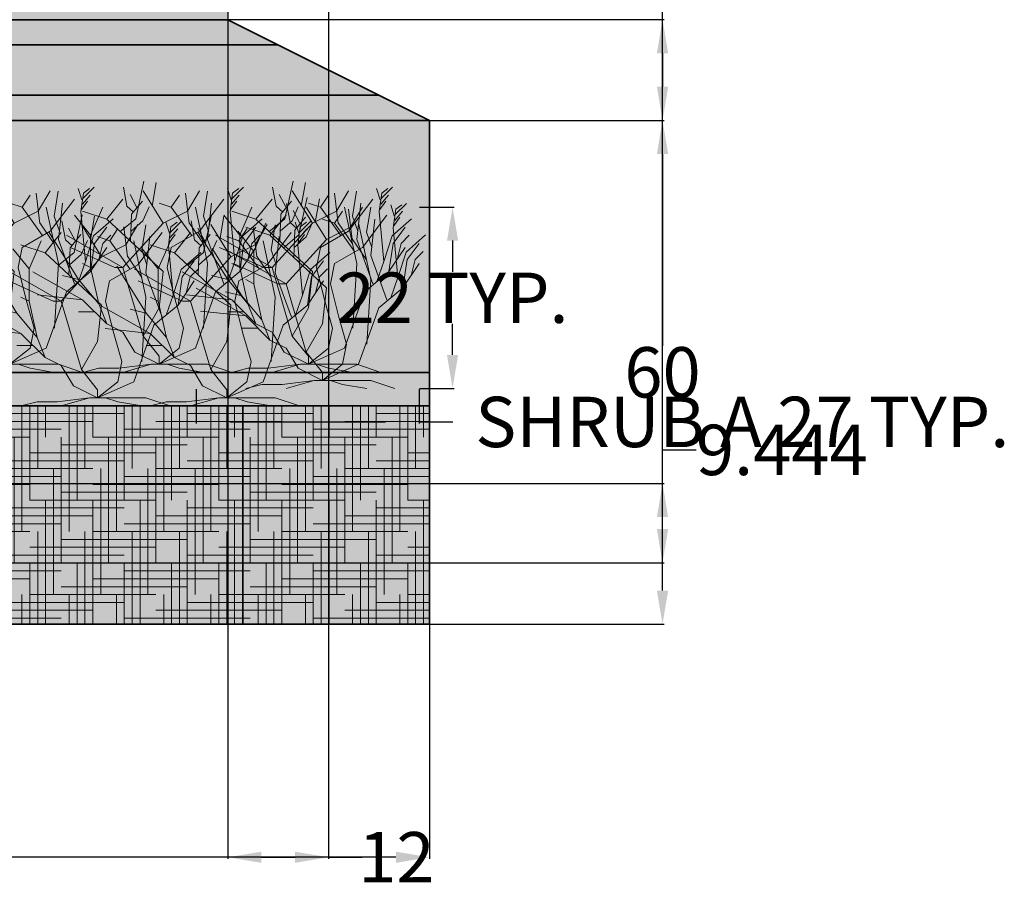
# Model space of a CAD drawing. Units: inches. Extents: x 221 to 874, y 171 to 738.
# Tile 9 of 11: x 756 to 874, y 171 to 275. Entities that reach past the tile are written whole.
import ezdxf

# ---------------------------------------------------------------- set-up
doc = ezdxf.new("R2010")
doc.units = ezdxf.units.IN
doc.header["$MEASUREMENT"] = 0
for name, color, linetype, lineweight in [('A-ANNO-DIMS', 2, 'Continuous', 18), ('A-ELEV', 7, 'Continuous', 35), ('A-ELEV-PATT', 8, 'Continuous', 13), ('L-PLNT', 3, 'Continuous', 13)]:
    doc.layers.add(name, color=color, linetype=linetype, lineweight=lineweight)
doc.styles.get("Standard").update_dxf_attribs({"font": 'arial.ttf'})
doc.dimstyles.get("Standard").update_dxf_attribs({"dimtxt": 6, "dimasz": 4, "dimexe": 0.18, "dimexo": 0.0625, "dimgap": 0.09, "dimtad": 0, "dimtih": 1, "dimtoh": 1, "dimdec": 0, "dimzin": 0, "dimdsep": 46, "dimlunit": 3, "dimtxsty": 'Standard', "dimcen": 0.09, "dimadec": 0, "dimazin": 0, "dimtfac": 1, "dimtdec": 0, "dimtofl": 0, "dimtmove": 0, "dimatfit": 3, "dimfxl": 1, "dimtolj": 1, "dimtzin": 0, "dimarcsym": 0})

# ---------------------------------------------------------------- blocks, each defined once
blk = doc.blocks.new('SHRUB-A')
for p, q in [((15.5, 17.76), (13.1, 21.6)), ((18.38, 19.2), (19.82, 21.6)), ((8.78, 18.24), (10.7, 20.64)), ((19.82, 16.8), (22.7, 20.64)), ((8.78, 18.24), (5.9, 19.2)), ((6.86, 16.32), (8.3, 19.68)), ((15.5, 17.76), (18.38, 19.2)), ((6.86, 16.32), (4.94, 18.72)), ((15.5, 12), (8.78, 18.24)), ((10.7, 12.48), (15.5, 17.76)), ((5.42, 11.04), (1.91, 16.66)), ((16.46, 14.88), (19.82, 16.8)), ((25.1, 15.36), (26.54, 17.28)), ((10.7, 12.48), (3.98, 16.32)), ((6.86, 12.48), (6.86, 16.32)), ((24.62, 12), (25.1, 15.36)), ((9.74, 12.48), (4.46, 14.88)), ((15.98, 12.48), (16.46, 14.88)), ((24.62, 12), (26.54, 14.88)), ((6.86, 12.48), (5.9, 12.96)), ((5.9, 8.64), (0, 11.96)), ((7.82, 8.16), (6.86, 12.48)), ((10.7, 12.48), (9.74, 12.48)), ((13.1, 4.32), (10.7, 12.48)), ((15.02, 7.68), (15.5, 12)), ((16.94, 8.64), (15.98, 12.48)), ((21.74, 9.6), (24.62, 12)), ((5.42, 11.04), (3.5, 11.52)), ((7.82, 8.16), (5.42, 11.04)), ((19.34, 2.88), (21.74, 9.6)), ((5.9, 8.64), (0.53, 9.22)), ((8.78, 5.76), (5.9, 8.64)), ((17.9, 5.28), (16.94, 8.64)), ((8.78, 5.76), (7.82, 8.16)), ((13.1, 4.32), (15.02, 7.68)), ((10.7, 4.8), (8.78, 5.76)), ((12.14, 2.4), (10.7, 4.8)), ((17.42, 2.88), (17.9, 5.28)), ((15.02, 1.92), (13.1, 4.32)), ((15.02, 0.96), (12.14, 2.4)), ((15.02, 0.96), (19.34, 2.88)), ((15.02, 0.96), (17.42, 2.88)), ((15.02, 0.96), (15.02, 1.92)), ((15.02, 0.96), (20.78, 0.96)), ((20.78, 0.96), (23.66, 0))]:
    blk.add_line(p, q)
blk = doc.blocks.new('GRASS-TUFT')
for p, q in [((0.58, 10.54), (1.31, 11.09)), ((0.28, 8.35), (0.58, 10.54)), ((0.83, 2.4), (0.28, 8.35)), ((1.8, 5.45), (4.12, 7.49)), ((0.83, 2.4), (1.8, 5.45)), ((0, 0), (0.83, 2.4))]:
    blk.add_line(p, q)
blk = doc.blocks.new('SHRUB-B')
for p, q in [((15.5, 17.76), (13.1, 21.6)), ((18.38, 19.2), (19.82, 21.6)), ((8.78, 18.24), (10.7, 20.64)), ((19.82, 16.8), (22.7, 20.64)), ((8.78, 18.24), (5.9, 19.2)), ((6.86, 16.32), (8.3, 19.68)), ((15.5, 17.76), (18.38, 19.2)), ((6.86, 16.32), (4.94, 18.72)), ((15.5, 12), (8.78, 18.24)), ((10.7, 12.48), (15.5, 17.76)), ((5.42, 11.04), (1.91, 16.66)), ((16.46, 14.88), (19.82, 16.8)), ((25.1, 15.36), (26.54, 17.28)), ((10.7, 12.48), (3.98, 16.32)), ((6.86, 12.48), (6.86, 16.32)), ((24.62, 12), (25.1, 15.36)), ((9.74, 12.48), (4.46, 14.88)), ((15.98, 12.48), (16.46, 14.88)), ((24.62, 12), (26.54, 14.88)), ((6.86, 12.48), (5.9, 12.96)), ((5.9, 8.64), (0, 11.96)), ((7.82, 8.16), (6.86, 12.48)), ((10.7, 12.48), (9.74, 12.48)), ((13.1, 4.32), (10.7, 12.48)), ((15.02, 7.68), (15.5, 12)), ((16.94, 8.64), (15.98, 12.48)), ((21.74, 9.6), (24.62, 12)), ((5.42, 11.04), (3.5, 11.52)), ((7.82, 8.16), (5.42, 11.04)), ((19.34, 2.88), (21.74, 9.6)), ((5.9, 8.64), (0.53, 9.22)), ((8.78, 5.76), (5.9, 8.64)), ((17.9, 5.28), (16.94, 8.64)), ((8.78, 5.76), (7.82, 8.16)), ((13.1, 4.32), (15.02, 7.68)), ((10.7, 4.8), (8.78, 5.76)), ((12.14, 2.4), (10.7, 4.8)), ((17.42, 2.88), (17.9, 5.28)), ((15.02, 1.92), (13.1, 4.32)), ((15.02, 0.96), (12.14, 2.4)), ((15.02, 0.96), (19.34, 2.88)), ((15.02, 0.96), (17.42, 2.88)), ((15.02, 0.96), (15.02, 1.92)), ((15.02, 0.96), (20.78, 0.96)), ((20.78, 0.96), (23.66, 0)), ((25.58, 0.48), (23.66, 0)), ((27.98, 0.48), (25.58, 0.48)), ((31.82, 0.96), (27.98, 0.48)), ((31.82, 0.96), (28.46, 0)), ((31.82, 0.96), (33.74, 0.96)), ((33.74, 0.96), (35.18, 0.48)), ((35.18, 0.48), (38.06, 0))]:
    blk.add_line(p, q)
blk = doc.blocks.new('GRASS-SPRIG')
for p, q in [((1.44, 3.36), (2.4, 4.8)), ((1.44, 3.36), (0, 3.84)), ((3.84, 0), (1.44, 3.36))]:
    blk.add_line(p, q)
blk = doc.blocks.new('*D14')
at = {"layer": 'A-ANNO-DIMS', "color": 0, "lineweight": -2, "transparency": 16777216}
for p, q in [((777.31, 230.73), (777.31, 226.63)), ((803.85, 230.73), (803.85, 226.63)), ((781.31, 226.81), (799.85, 226.81)), ((803.85, 226.81), (807.85, 226.81))]:
    blk.add_line(p, q, dxfattribs=at)
at = {"layer": 'A-ANNO-DIMS', "color": 0, "transparency": 16777216}
for points in [[(781.31, 227.48), (781.31, 226.15), (777.31, 226.81)], [(799.85, 227.48), (799.85, 226.15), (803.85, 226.81)]]:
    blk.add_solid(points, dxfattribs=at)
at = {"layer": 'Defpoints', "color": 0, "transparency": 16777216}
for p in [(777.31, 230.8), (803.85, 230.8), (803.85, 226.81)]:
    blk.add_point(p, dxfattribs=at)
at = {"layer": 'A-ANNO-DIMS', "color": 0, "transparency": 16777216, "insert": (842.33, 226.81), "char_height": 6, "attachment_point": 5}
blk.add_mtext('\\A1;SHRUB A 27 TYP.', dxfattribs=at)
blk = doc.blocks.new('*D15')
at = {"layer": 'A-ANNO-DIMS', "color": 0, "lineweight": -2, "transparency": 16777216}
for p, q in [((803.91, 252.4), (808.01, 252.4)), ((807.83, 248.4), (807.83, 244.7)), ((807.83, 234.8), (807.83, 238.49)), ((803.91, 230.8), (808.01, 230.8))]:
    blk.add_line(p, q, dxfattribs=at)
at = {"layer": 'A-ANNO-DIMS', "color": 0, "transparency": 16777216}
for points in [[(807.17, 248.4), (808.5, 248.4), (807.83, 252.4)], [(807.17, 234.8), (808.5, 234.8), (807.83, 230.8)]]:
    blk.add_solid(points, dxfattribs=at)
at = {"layer": 'Defpoints', "color": 0, "transparency": 16777216}
for p in [(803.85, 252.4), (807.83, 252.4), (803.85, 230.8)]:
    blk.add_point(p, dxfattribs=at)
at = {"layer": 'A-ANNO-DIMS', "color": 0, "transparency": 16777216, "insert": (807.83, 241.6), "char_height": 6, "attachment_point": 5}
blk.add_mtext('\\A1;22 TYP.', dxfattribs=at)
blk = doc.blocks.new('*D20')
at = {"layer": 'A-ANNO-DIMS', "color": 0, "lineweight": -2, "transparency": 16777216}
for p, q in [((313.08, 202.65), (313.08, 174.79)), ((805.08, 202.65), (805.08, 174.79)), ((317.08, 174.97), (552.27, 174.97)), ((801.08, 174.97), (565.89, 174.97))]:
    blk.add_line(p, q, dxfattribs=at)
at = {"layer": 'A-ANNO-DIMS', "color": 0, "transparency": 16777216}
for points in [[(317.08, 175.63), (317.08, 174.3), (313.08, 174.97)], [(801.08, 175.63), (801.08, 174.3), (805.08, 174.97)]]:
    blk.add_solid(points, dxfattribs=at)
at = {"layer": 'Defpoints', "color": 0, "transparency": 16777216}
for p in [(313.08, 202.72), (805.08, 202.72), (805.08, 174.97)]:
    blk.add_point(p, dxfattribs=at)
at = {"layer": 'A-ANNO-DIMS', "color": 0, "transparency": 16777216, "insert": (559.08, 174.97), "char_height": 6, "attachment_point": 5}
blk.add_mtext('\\A1;492', dxfattribs=at)
blk = doc.blocks.new('*D21')
at = {"layer": 'A-ANNO-DIMS', "color": 0, "lineweight": -2, "transparency": 16777216}
for p, q in [((541.14, 706.72), (833.01, 706.72)), ((832.83, 702.72), (832.83, 457.87)), ((832.83, 206.72), (832.83, 451.56)), ((805.14, 202.72), (833.01, 202.72))]:
    blk.add_line(p, q, dxfattribs=at)
at = {"layer": 'A-ANNO-DIMS', "color": 0, "transparency": 16777216}
for points in [[(832.16, 702.72), (833.5, 702.72), (832.83, 706.72)], [(832.16, 206.72), (833.5, 206.72), (832.83, 202.72)]]:
    blk.add_solid(points, dxfattribs=at)
at = {"layer": 'Defpoints', "color": 0, "transparency": 16777216}
for p in [(541.08, 706.72), (832.83, 706.72), (805.08, 202.72)]:
    blk.add_point(p, dxfattribs=at)
at = {"layer": 'A-ANNO-DIMS', "color": 0, "transparency": 16777216, "insert": (832.83, 454.72), "char_height": 6, "attachment_point": 5}
blk.add_mtext('\\A1;504', dxfattribs=at)
blk = doc.blocks.new('*D46')
at = {"layer": 'A-ANNO-DIMS', "color": 0, "lineweight": -2, "transparency": 16777216}
for p, q in [((793.08, 430.65), (793.08, 174.79)), ((781.08, 418.65), (781.08, 174.79)), ((785.08, 174.97), (789.08, 174.97)), ((793.08, 174.97), (797.08, 174.97))]:
    blk.add_line(p, q, dxfattribs=at)
at = {"layer": 'A-ANNO-DIMS', "color": 0, "transparency": 16777216}
for points in [[(785.08, 175.63), (785.08, 174.3), (781.08, 174.97)], [(789.08, 175.63), (789.08, 174.3), (793.08, 174.97)]]:
    blk.add_solid(points, dxfattribs=at)
at = {"layer": 'Defpoints', "color": 0, "transparency": 16777216}
for p in [(793.08, 430.72), (781.08, 418.72), (793.08, 174.97)]:
    blk.add_point(p, dxfattribs=at)
at = {"layer": 'A-ANNO-DIMS', "color": 0, "transparency": 16777216, "insert": (801.15, 174.97), "char_height": 6, "attachment_point": 5}
blk.add_mtext('\\A1;12', dxfattribs=at)
blk = doc.blocks.new('*D62')
at = {"layer": 'A-ANNO-DIMS', "color": 0, "lineweight": -2, "transparency": 16777216}
for p, q in [((805.14, 262.72), (833.01, 262.72)), ((832.83, 258.72), (832.83, 235.87)), ((832.83, 206.72), (832.83, 229.56)), ((805.14, 202.72), (833.01, 202.72))]:
    blk.add_line(p, q, dxfattribs=at)
at = {"layer": 'A-ANNO-DIMS', "color": 0, "transparency": 16777216}
for points in [[(832.16, 258.72), (833.5, 258.72), (832.83, 262.72)], [(832.16, 206.72), (833.5, 206.72), (832.83, 202.72)]]:
    blk.add_solid(points, dxfattribs=at)
at = {"layer": 'Defpoints', "color": 0, "transparency": 16777216}
for p in [(805.08, 262.72), (832.83, 262.72), (805.08, 202.72)]:
    blk.add_point(p, dxfattribs=at)
at = {"layer": 'A-ANNO-DIMS', "color": 0, "transparency": 16777216, "insert": (832.83, 232.72), "char_height": 6, "attachment_point": 5}
blk.add_mtext('\\A1;60', dxfattribs=at)
blk = doc.blocks.new('*D63')
at = {"layer": 'A-ANNO-DIMS', "color": 0, "lineweight": -2, "transparency": 16777216}
for p, q in [((832.83, 274.72), (832.83, 278.72)), ((832.83, 278.72), (836.83, 278.72)), ((781.14, 274.72), (833.01, 274.72)), ((832.83, 266.72), (832.83, 270.72)), ((805.14, 262.72), (833.01, 262.72))]:
    blk.add_line(p, q, dxfattribs=at)
at = {"layer": 'A-ANNO-DIMS', "color": 0, "transparency": 16777216}
for points in [[(832.16, 270.72), (833.5, 270.72), (832.83, 274.72)], [(832.16, 266.72), (833.5, 266.72), (832.83, 262.72)]]:
    blk.add_solid(points, dxfattribs=at)
at = {"layer": 'Defpoints', "color": 0, "transparency": 16777216}
for p in [(781.08, 274.72), (832.83, 274.72), (805.08, 262.72)]:
    blk.add_point(p, dxfattribs=at)
at = {"layer": 'A-ANNO-DIMS', "color": 0, "transparency": 16777216, "insert": (840.9, 278.72), "char_height": 6, "attachment_point": 5}
blk.add_mtext('\\A1;12', dxfattribs=at)
blk = doc.blocks.new('*D64')
at = {"layer": 'A-ANNO-DIMS', "color": 0, "lineweight": -2, "transparency": 16777216}
for p, q in [((832.83, 284.72), (832.83, 288.72)), ((832.83, 288.72), (836.83, 288.72)), ((705.97, 280.72), (833.01, 280.72)), ((781.14, 274.72), (833.01, 274.72)), ((832.83, 270.72), (832.83, 266.72))]:
    blk.add_line(p, q, dxfattribs=at)
at = {"layer": 'A-ANNO-DIMS', "color": 0, "transparency": 16777216}
for points in [[(832.16, 284.72), (833.5, 284.72), (832.83, 280.72)], [(832.16, 270.72), (833.5, 270.72), (832.83, 274.72)]]:
    blk.add_solid(points, dxfattribs=at)
at = {"layer": 'Defpoints', "color": 0, "transparency": 16777216}
for p in [(705.91, 280.72), (832.83, 280.72), (781.08, 274.72)]:
    blk.add_point(p, dxfattribs=at)
at = {"layer": 'A-ANNO-DIMS', "color": 0, "transparency": 16777216, "insert": (838.9, 288.72), "char_height": 6, "attachment_point": 5}
blk.add_mtext('\\A1;6', dxfattribs=at)
blk = doc.blocks.new('*D70')
at = {"layer": 'A-ANNO-DIMS', "color": 0, "lineweight": -2, "transparency": 16777216}
for p, q in [((625.96, 229.65), (625.96, 174.79)), ((805.08, 202.65), (805.08, 174.79)), ((629.96, 174.97), (703.29, 174.97)), ((801.08, 174.97), (727.75, 174.97))]:
    blk.add_line(p, q, dxfattribs=at)
at = {"layer": 'A-ANNO-DIMS', "color": 0, "transparency": 16777216}
for points in [[(629.96, 175.63), (629.96, 174.3), (625.96, 174.97)], [(801.08, 175.63), (801.08, 174.3), (805.08, 174.97)]]:
    blk.add_solid(points, dxfattribs=at)
at = {"layer": 'Defpoints', "color": 0, "transparency": 16777216}
for p in [(625.96, 229.72), (805.08, 202.72), (805.08, 174.97)]:
    blk.add_point(p, dxfattribs=at)
at = {"layer": 'A-ANNO-DIMS', "color": 0, "transparency": 16777216, "insert": (715.52, 174.97), "char_height": 6, "attachment_point": 5}
blk.add_mtext('\\A1;179.12', dxfattribs=at)
blk = doc.blocks.new('*D72')
at = {"layer": 'A-ANNO-DIMS', "color": 0, "lineweight": -2, "transparency": 16777216}
for p, q in [((832.83, 219.48), (832.83, 223.48)), ((832.83, 223.48), (836.83, 223.48)), ((706.95, 219.48), (833.01, 219.48)), ((832.83, 214.04), (832.83, 215.48)), ((706.95, 210.04), (833.01, 210.04))]:
    blk.add_line(p, q, dxfattribs=at)
at = {"layer": 'A-ANNO-DIMS', "color": 0, "transparency": 16777216}
for points in [[(832.16, 215.48), (833.5, 215.48), (832.83, 219.48)], [(832.16, 214.04), (833.5, 214.04), (832.83, 210.04)]]:
    blk.add_solid(points, dxfattribs=at)
at = {"layer": 'Defpoints', "color": 0, "transparency": 16777216}
for p in [(706.89, 219.48), (832.83, 219.48), (706.89, 210.04)]:
    blk.add_point(p, dxfattribs=at)
at = {"layer": 'A-ANNO-DIMS', "color": 0, "transparency": 16777216, "insert": (847.03, 223.48), "char_height": 6, "attachment_point": 5}
blk.add_mtext('\\A1;9.444', dxfattribs=at)

msp = doc.modelspace()

# ---------------------------------------------------------------- hatches: boundary and pattern name
at = {"layer": 'A-ELEV-PATT'}
h = msp.add_hatch(color=256, dxfattribs=at)
h.dxf.hatch_style = 1
h.paths.add_polyline_path([(349.0786, 286.1996), (313.0786, 286.1996), (313.0786, 232.7164), (349.0786, 232.7164)])
h.paths.add_polyline_path([(464.0786, 286.1996), (406.0786, 286.1996), (406.0786, 232.7164), (464.0786, 232.7164)])
h.paths.add_polyline_path([(541.0786, 286.1996), (493.0786, 286.1996), (493.0786, 232.7164), (541.0786, 232.7164)])
h.paths.add_polyline_path([(541.0786, 370.7164), (493.0786, 370.7164), (493.0786, 286.1996), (541.0786, 286.1996)])
h.paths.add_polyline_path([(464.0786, 370.7164), (406.0786, 370.7164), (406.0786, 286.1996), (464.0786, 286.1996)])
h.paths.add_polyline_path([(349.0786, 370.7164), (313.0786, 370.7164), (313.0786, 286.1996), (349.0786, 286.1996)])
h.paths.add_polyline_path([(349.0786, 454.7164), (313.0786, 454.7164), (313.0786, 370.7164), (349.0786, 370.7164)])
h.paths.add_polyline_path([(464.0786, 454.7164), (406.0786, 454.7164), (406.0786, 370.7164), (464.0786, 370.7164)])
h.paths.add_polyline_path([(541.0786, 418.7164), (541.0786, 454.7164), (493.0786, 454.7164), (493.0786, 370.7164), (541.0786, 370.7164)])
h.paths.add_polyline_path([(541.0786, 550.7164), (493.0786, 550.7164), (493.0786, 454.7164), (541.0786, 454.7164)])
h.paths.add_polyline_path([(464.0786, 550.7164), (406.0786, 550.7164), (406.0786, 454.7164), (464.0786, 454.7164)])
h.paths.add_polyline_path([(349.0786, 550.7164), (313.0786, 550.7164), (313.0786, 454.7164), (349.0786, 454.7164)])
h.paths.add_polyline_path([(349.0786, 586.7164), (313.0786, 586.7164), (313.0786, 550.7164), (349.0786, 550.7164)])
h.paths.add_polyline_path([(464.0786, 586.7164), (406.0786, 586.7164), (406.0786, 550.7164), (464.0786, 550.7164)])
h.paths.add_polyline_path([(541.0786, 574.7164), (541.0786, 586.7164), (493.0786, 586.7164), (493.0786, 550.7164), (541.0786, 550.7164)])
h.paths.add_polyline_path([(541.0786, 670.7164), (493.0786, 670.7164), (493.0786, 586.7164), (541.0786, 586.7164)])
h.paths.add_polyline_path([(464.0786, 670.7164), (406.0786, 670.7164), (406.0786, 586.7164), (464.0786, 586.7164)])
h.paths.add_polyline_path([(349.0786, 670.7164), (313.0786, 670.7164), (313.0786, 586.7164), (349.0786, 586.7164)])
h.paths.add_polyline_path([(406.0786, 706.7164), (313.0786, 706.7164), (313.0786, 670.7164), (349.0786, 670.7164), (406.0786, 670.7164)])
h.paths.add_polyline_path([(464.0786, 706.7164), (406.0786, 706.7164), (406.0786, 670.7164), (464.0786, 670.7164)])
h.paths.add_polyline_path([(541.0786, 706.7164), (493.0786, 706.7164), (493.0786, 688.7164), (493.0786, 670.7164), (541.0786, 670.7164)])
h.paths.add_polyline_path([(660.0786, 610.7164), (541.0786, 610.7164), (541.0786, 586.7164), (541.0786, 574.7164), (660.0786, 574.7164)])
h.paths.add_polyline_path([(781.0786, 610.7164), (660.0786, 610.7164), (660.0786, 574.7164), (769.0786, 574.7164), (781.0786, 574.7164)])
h.paths.add_polyline_path([(781.0786, 574.7164), (769.0786, 574.7164), (769.0786, 476.1199), (781.0786, 476.1199)])
h.paths.add_polyline_path([(781.0786, 476.1199), (769.0786, 476.1199), (769.0786, 457.7164), (781.0786, 457.7164)])
h.paths.add_polyline_path([(781.0786, 377.1023), (705.9097, 377.1023), (705.9097, 286.1996), (781.0786, 286.1996)])
h.paths.add_polyline_path([(741.9618, 338.8486), (756.9618, 338.8486), (756.9618, 329.8486), (741.9618, 329.8486)], flags=16)
h.paths.add_polyline_path([(648.9097, 377.1023), (598.0786, 377.1023), (598.0786, 286.1996), (648.9097, 286.1996)])
h.paths.add_polyline_path([(781.0786, 286.1996), (705.9097, 286.1996), (705.9097, 280.7164), (648.9097, 280.7164), (648.9097, 286.1996), (598.0786, 286.1996), (598.0786, 280.7164), (550.0786, 280.7164), (550.0786, 286.1996), (541.0786, 286.1996), (541.0786, 274.7164), (781.0786, 274.7164)])
h.paths.add_polyline_path([(660.0786, 562.7164), (546.3477, 562.7164), (546.3477, 457.7164), (660.0786, 457.7164)])
h = msp.add_hatch(color=256, dxfattribs=at)
h.set_gradient(color1=(99, 100, 102), color2=(169, 160, 132), name='INVCYLINDER')
h.paths.add_polyline_path([(541.0786, 274.7164), (541.0786, 271.7164), (787.0786, 271.7164), (781.0786, 274.7164)])
h = msp.add_hatch(color=256, dxfattribs=at)
h.paths.add_polyline_path([(787.0786, 271.7164), (541.0786, 271.7164), (541.0786, 265.7164), (799.0786, 265.7164)])
h.paths.add_polyline_path([(631.9596, 262.7164), (541.0786, 262.7164), (541.0786, 256.7164), (631.9596, 256.7164)])
h.paths.add_polyline_path([(631.9596, 253.7164), (541.0786, 253.7164), (541.0786, 247.7164), (631.9596, 247.7164)])
h.paths.add_polyline_path([(631.9596, 244.7164), (541.0786, 244.7164), (541.0786, 238.7164), (631.9596, 238.7164)])
h.paths.add_polyline_path([(631.9596, 235.7164), (541.0786, 235.7164), (541.0786, 229.7164), (625.9596, 229.7164), (625.9596, 232.7164), (631.9596, 232.7164)])
h.paths.add_polyline_path([(630.2472, 217.7164), (538.2859, 217.7164), (538.2859, 211.7164), (634.5124, 211.7164), (634.5123, 211.7326)], flags=17)
h.paths.add_polyline_path([(634.5396, 208.7164), (538.2859, 208.7164), (538.2859, 202.7164), (638.8162, 202.7164)])
h = msp.add_hatch(color=256, dxfattribs=at)
h.set_gradient(color1=(99, 100, 102), color2=(248, 246, 176), name='CYLINDER')
h.paths.add_polyline_path([(805.0786, 262.7164), (799.0786, 265.7164), (541.0786, 265.7164), (541.0786, 262.7164)])
for points in [[(631.9596, 262.7164), (631.9596, 232.7164), (805.0786, 232.7164), (805.0786, 262.7164)], [(805.0786, 228.7164), (805.0786, 232.7164), (625.9596, 232.7164), (625.9596, 228.7164)]]:
    msp.add_hatch(color=256, dxfattribs=at).paths.add_polyline_path(points)
h = msp.add_hatch(color=256, dxfattribs=at)
h.set_gradient(color1=(99, 100, 102), color2=(91, 91, 91), rotation=180, name='INVCURVED')
h.paths.add_polyline_path([(680.047, 219.4807), (680.047, 228.7164), (656.1863, 228.7164), (656.1863, 202.7164), (680.047, 202.7164), (680.047, 210.037), (660.2585, 210.037), (660.2585, 219.4807)])
h.paths.add_polyline_path([(662.2585, 217.4807), (662.2585, 212.037), (680.047, 212.037), (680.047, 217.4807)], flags=17)
h.paths.add_polyline_path([(782.8632, 202.7164), (782.8632, 228.7164), (735.4784, 228.7164), (735.4784, 202.7164)])
h = msp.add_hatch(dxfattribs=at)
h.set_pattern_fill('HOUND', color=256, scale=15, style=0)
h.paths.add_polyline_path([(782.8632, 228.7164), (735.4784, 228.7164), (735.4784, 202.7164), (782.8632, 202.7164)])
h = msp.add_hatch(color=256, dxfattribs=at)
h.set_gradient(color1=(147, 149, 152), color2=(99, 100, 102), name='CURVED')
h.paths.add_polyline_path([(805.0786, 228.7164), (782.8632, 228.7164), (782.8632, 202.7164), (805.0786, 202.7164)])
h = msp.add_hatch(dxfattribs=at)
h.set_pattern_fill('HOUND', color=256, scale=15, style=0)
h.paths.add_polyline_path([(805.0786, 228.7164), (782.8632, 228.7164), (782.8632, 202.7164), (805.0786, 202.7164)])

# ---------------------------------------------------------------- linework, layer by layer
at = {"layer": 'A-ELEV'}
for p, q in [((781.0786, 274.7164), (541.0786, 274.7164)), ((781.0786, 274.7164), (805.0786, 262.7164)), ((787.0786, 271.7164), (541.0786, 271.7164)), ((799.0786, 265.7164), (541.0786, 265.7164)), ((805.0786, 262.7164), (541.0786, 262.7164)), ((805.0786, 262.7164), (805.0786, 202.7164)), ((805.0786, 232.7164), (625.9596, 232.7164)), ((805.0786, 228.7164), (625.9596, 228.7164)), ((782.8632, 202.7164), (782.8632, 228.7164)), ((805.0786, 202.7164), (313.0786, 202.7164))]:
    msp.add_line(p, q, dxfattribs=at)
at = {"layer": 'L-PLNT'}
for p, q in [((763.2755, 254.6044), (763.7025, 253.2744)), ((763.8245, 253.4304), (765.1675, 254.7604)), ((769.0725, 252.4914), (768.6455, 254.7604)), ((770.1105, 251.0054), (771.0865, 255.4654)), ((772.0635, 252.4914), (772.5515, 255.3084)), ((781.0355, 254.6044), (781.4625, 253.2744)), ((781.5845, 253.4304), (782.9275, 254.7604)), ((786.8325, 252.4914), (786.4055, 254.7604)), ((787.8705, 251.0054), (788.8465, 255.4654)), ((789.8235, 252.4914), (790.3115, 255.3084)), ((798.7955, 254.6044), (799.2225, 253.2744)), ((799.3445, 253.4304), (800.6875, 254.7604)), ((758.6975, 250.4574), (758.2705, 254.0564)), ((760.4065, 251.3184), (760.8955, 254.2914)), ((763.7635, 252.7264), (764.6795, 253.8214)), ((766.6635, 250.9564), (768.5835, 253.3564)), ((770.2635, 252.3354), (769.4395, 253.9004)), ((773.3835, 250.4764), (770.9835, 254.3164)), ((776.4575, 250.4574), (776.0305, 254.0564)), ((776.2635, 251.9164), (777.7035, 254.3164)), ((777.7035, 249.5164), (780.5835, 253.3564)), ((778.1665, 251.3184), (778.6555, 254.2914)), ((781.5235, 252.7264), (782.4395, 253.8214)), ((784.4235, 250.9564), (786.3435, 253.3564)), ((788.0235, 252.3354), (787.1995, 253.9004)), ((791.1435, 250.4764), (788.7435, 254.3164)), ((789.5395, 249.0854), (790.5155, 253.5454)), ((791.4925, 250.5714), (791.9805, 253.3884)), ((794.2175, 250.4574), (793.7905, 254.0564)), ((794.0235, 251.9164), (795.4635, 254.3164)), ((795.4635, 249.5164), (798.3435, 253.3564)), ((795.9265, 251.3184), (796.4155, 254.2914)), ((799.2835, 252.7264), (800.1995, 253.8214)), ((760.9035, 245.6764), (759.4635, 252.3964)), ((760.9035, 248.5564), (761.3835, 252.8764)), ((763.6415, 252.1004), (764.3735, 253.1174)), ((764.7435, 249.0364), (766.1835, 252.3964)), ((769.8665, 251.7874), (769.0725, 252.4914)), ((769.6225, 251.5524), (770.9035, 253.1174)), ((770.9645, 250.7704), (771.6975, 252.4134)), ((778.6635, 245.6764), (777.2235, 252.3964)), ((778.6635, 248.5564), (779.1435, 252.8764)), ((781.4015, 252.1004), (782.1335, 253.1174)), ((782.5035, 249.0364), (783.9435, 252.3964)), ((787.6265, 251.7874), (786.8325, 252.4914)), ((787.3825, 251.5524), (788.6635, 253.1174)), ((788.5015, 250.5714), (788.0745, 252.8404)), ((788.7245, 250.7704), (789.4575, 252.4134)), ((796.4235, 245.6764), (794.9835, 252.3964)), ((795.8865, 248.5374), (795.4595, 252.1364)), ((796.4235, 248.5564), (796.9035, 252.8764)), ((797.5955, 249.3984), (798.0845, 252.3714)), ((799.1615, 252.1004), (799.8935, 253.1174)), ((800.4645, 252.6844), (800.8915, 251.3544)), ((801.0135, 251.5104), (802.3565, 252.8404)), ((761.0175, 249.5184), (760.4065, 251.3184)), ((762.7772, 247.0054), (763.7532, 251.4654)), ((764.7435, 249.0364), (762.8235, 251.4364)), ((766.6635, 250.9564), (763.7835, 251.9164)), ((764.7302, 248.4914), (765.2182, 251.3084)), ((773.3835, 244.7164), (766.6635, 250.9564)), ((768.2185, 249.4404), (770.1105, 251.0054)), ((769.5005, 248.3444), (769.6225, 251.5524)), ((773.3835, 250.4764), (776.2635, 251.9164)), ((778.7775, 249.5184), (778.1665, 251.3184)), ((778.167, 247.0054), (779.143, 251.4654)), ((780.12, 248.4914), (780.608, 251.3084)), ((782.5035, 249.0364), (780.5835, 251.4364)), ((784.4235, 250.9564), (781.5435, 251.9164)), ((791.1435, 244.7164), (784.4235, 250.9564)), ((785.9785, 249.4404), (787.8705, 251.0054)), ((787.2605, 248.3444), (787.3825, 251.5524)), ((789.6925, 250.4154), (788.8685, 251.9804)), ((789.0515, 249.6324), (790.3325, 251.1974)), ((791.1435, 250.4764), (794.0235, 251.9164)), ((796.5375, 249.5184), (795.9265, 251.3184)), ((798.0925, 246.6364), (798.5725, 250.9564)), ((800.8305, 250.1804), (801.5625, 251.1974)), ((800.9525, 250.8064), (801.8685, 251.9014)), ((760.4065, 248.0314), (758.6975, 250.5354)), ((761.7392, 248.4914), (761.3122, 250.7604)), ((762.9302, 248.3354), (762.1062, 249.9004)), ((768.5835, 245.1964), (773.3835, 250.4764)), ((769.1242, 246.4574), (768.6972, 250.0564)), ((769.5615, 249.5184), (770.9645, 250.7704)), ((770.8332, 247.3184), (771.3222, 250.2914)), ((773.7022, 250.6044), (774.1292, 249.2744)), ((774.1902, 248.7264), (775.1062, 249.8214)), ((774.2512, 249.4304), (775.5942, 250.7604)), ((778.1665, 248.0314), (776.4575, 250.5354)), ((777.129, 248.4914), (776.702, 250.7604)), ((778.32, 248.3354), (777.496, 249.9004)), ((782.9835, 248.0764), (784.4235, 249.9964)), ((784.514, 246.4574), (784.087, 250.0564)), ((786.223, 247.3184), (786.712, 250.2914)), ((786.3435, 245.1964), (791.1435, 250.4764)), ((787.3215, 249.5184), (788.7245, 250.7704)), ((789.2955, 249.8674), (788.5015, 250.5714)), ((789.092, 250.6044), (789.519, 249.2744)), ((789.58, 248.7264), (790.496, 249.8214)), ((789.641, 249.4304), (790.984, 250.7604)), ((790.3935, 248.8504), (791.1265, 250.4934)), ((795.9265, 248.0314), (794.2175, 250.5354)), ((798.0925, 243.7564), (796.6525, 250.4764)), ((800.7435, 248.0764), (802.1835, 249.9964)), ((763.3035, 243.7564), (759.7885, 249.3714)), ((762.8235, 243.2764), (760.9035, 248.5564)), ((768.5835, 245.1964), (761.8635, 249.0364)), ((762.2892, 247.5524), (763.5702, 249.1174)), ((764.7435, 245.1964), (764.7435, 249.0364)), ((766.1835, 248.0764), (767.1435, 249.0364)), ((771.3302, 244.5564), (771.8102, 248.8764)), ((774.0682, 248.1004), (774.8002, 249.1174)), ((774.3435, 247.5964), (777.7035, 249.5164)), ((781.0635, 243.7564), (777.5485, 249.3714)), ((777.679, 247.5524), (778.96, 249.1174)), ((780.5835, 243.2764), (778.6635, 248.5564)), ((786.3435, 245.1964), (779.6235, 249.0364)), ((782.5035, 245.1964), (782.5035, 249.0364)), ((783.9435, 248.0764), (784.9035, 249.0364)), ((786.72, 244.5564), (787.2, 248.8764)), ((787.6475, 247.5204), (789.5395, 249.0854)), ((788.9295, 246.4244), (789.0515, 249.6324)), ((788.9905, 247.5984), (790.3935, 248.8504)), ((789.458, 248.1004), (790.19, 249.1174)), ((792.1035, 247.5964), (795.4635, 249.5164)), ((797.5955, 246.1114), (795.8865, 248.6154)), ((798.3435, 243.2764), (796.4235, 248.5564)), ((798.2065, 247.5984), (797.5955, 249.3984)), ((801.7035, 248.0764), (802.6635, 249.0364)), ((762.5332, 247.7874), (761.7392, 248.4914)), ((762.1672, 244.3444), (762.2892, 247.5524)), ((767.6235, 245.1964), (762.3435, 247.5964)), ((763.6312, 246.7704), (764.3642, 248.4134)), ((765.7035, 246.1564), (766.1835, 248.0764)), ((771.3302, 241.6764), (769.8902, 248.3964)), ((773.8635, 245.1964), (774.3435, 247.5964)), ((777.923, 247.7874), (777.129, 248.4914)), ((777.557, 244.3444), (777.679, 247.5524)), ((779.021, 246.7704), (779.754, 248.4134)), ((785.3835, 245.1964), (780.1035, 247.5964)), ((782.5035, 244.7164), (782.9835, 248.0764)), ((782.5035, 244.7164), (784.4235, 247.5964)), ((783.4635, 246.1564), (783.9435, 248.0764)), ((786.72, 241.6764), (785.28, 248.3964)), ((791.6235, 245.1964), (792.1035, 247.5964)), ((800.2635, 244.7164), (800.7435, 248.0764)), ((800.2635, 244.7164), (802.1835, 247.5964)), ((801.2235, 246.1564), (801.7035, 248.0764)), ((760.8852, 245.4404), (762.7772, 247.0054)), ((762.2282, 245.5184), (763.6312, 246.7704)), ((770.8332, 244.0314), (769.1242, 246.5354)), ((771.4442, 245.5184), (770.8332, 247.3184)), ((776.275, 245.4404), (778.167, 247.0054)), ((777.618, 245.5184), (779.021, 246.7704)), ((786.223, 244.0314), (784.514, 246.5354)), ((786.834, 245.5184), (786.223, 247.3184)), ((800.0125, 241.3564), (798.0925, 246.6364)), ((803.3725, 246.1564), (804.3325, 247.1164)), ((760.4235, 237.9964), (760.9035, 245.6764)), ((764.7435, 245.1964), (763.7835, 245.6764)), ((765.7035, 240.8764), (764.7435, 245.1964)), ((768.5835, 245.1964), (767.6235, 245.1964)), ((770.9835, 237.0364), (768.5835, 245.1964)), ((774.8235, 241.3564), (773.8635, 245.1964)), ((776.6102, 244.0764), (777.5702, 245.0364)), ((778.1835, 237.9964), (778.6635, 245.6764)), ((782.5035, 245.1964), (781.5435, 245.6764)), ((783.4635, 240.8764), (782.5035, 245.1964)), ((786.3435, 245.1964), (785.3835, 245.1964)), ((788.7435, 237.0364), (786.3435, 245.1964)), ((792.5835, 241.3564), (791.6235, 245.1964)), ((792, 244.0764), (792.96, 245.0364)), ((795.9435, 237.9964), (796.4235, 245.6764)), ((802.8925, 244.2364), (803.3725, 246.1564)), ((763.7835, 241.3564), (757.8805, 244.6774)), ((763.3035, 243.7564), (761.3835, 244.2364)), ((773.2502, 239.2764), (771.3302, 244.5564)), ((772.9035, 240.3964), (773.3835, 244.7164)), ((781.5435, 241.3564), (775.6405, 244.6774)), ((776.1302, 242.1564), (776.6102, 244.0764)), ((781.0635, 243.7564), (779.1435, 244.2364)), ((779.6235, 242.3164), (782.5035, 244.7164)), ((788.64, 239.2764), (786.72, 244.5564)), ((790.6635, 240.3964), (791.1435, 244.7164)), ((791.52, 242.1564), (792, 244.0764)), ((797.3835, 242.3164), (800.2635, 244.7164)), ((765.7035, 240.8764), (763.3035, 243.7564)), ((783.4635, 240.8764), (781.0635, 243.7564)), ((797.6125, 236.0764), (798.0925, 243.7564)), ((763.7835, 241.3564), (758.4155, 241.9384)), ((770.8502, 233.9964), (771.3302, 241.6764)), ((781.5435, 241.3564), (776.1755, 241.9384)), ((777.2235, 235.5964), (779.6235, 242.3164)), ((786.24, 233.9964), (786.72, 241.6764)), ((794.9835, 235.5964), (797.3835, 242.3164)), ((766.6635, 238.4764), (763.7835, 241.3564)), ((766.6635, 238.4764), (765.7035, 240.8764)), ((770.9835, 237.0364), (772.9035, 240.3964)), ((775.7835, 237.9964), (774.8235, 241.3564)), ((784.4235, 238.4764), (781.5435, 241.3564)), ((784.4235, 238.4764), (783.4635, 240.8764)), ((788.7435, 237.0364), (790.6635, 240.3964)), ((793.5435, 237.9964), (792.5835, 241.3564)), ((765.2235, 239.9164), (763.3035, 239.9164)), ((782.9835, 239.9164), (781.0635, 239.9164)), ((768.5835, 237.5164), (766.6635, 238.4764)), ((775.3035, 235.5964), (775.7835, 237.9964)), ((784.6525, 237.9964), (782.7325, 237.9964)), ((786.3435, 237.5164), (784.4235, 238.4764)), ((793.0635, 235.5964), (793.5435, 237.9964)), ((770.0235, 235.1164), (768.5835, 237.5164)), ((772.9035, 234.6364), (770.9835, 237.0364)), ((787.7835, 235.1164), (786.3435, 237.5164)), ((790.6635, 234.6364), (788.7435, 237.0364)), ((757.8902, 235.9164), (755.9702, 235.9164)), ((773.28, 235.9164), (771.36, 235.9164)), ((772.9035, 233.6764), (770.0235, 235.1164)), ((772.9035, 233.6764), (777.2235, 235.5964)), ((772.9035, 233.6764), (775.3035, 235.5964)), ((772.9035, 233.6764), (772.9035, 234.6364)), ((790.6635, 233.6764), (787.7835, 235.1164)), ((790.6635, 233.6764), (794.9835, 235.5964)), ((790.6635, 233.6764), (793.0635, 235.5964)), ((790.6635, 233.6764), (790.6635, 234.6364)), ((772.9035, 233.6764), (778.6635, 233.6764)), ((778.6635, 233.6764), (781.5435, 232.7164)), ((789.7035, 233.6764), (785.8635, 233.1964)), ((789.7035, 233.6764), (786.3435, 232.7164)), ((789.7035, 233.6764), (791.6235, 233.6764)), ((790.6635, 233.6764), (796.4235, 233.6764)), ((791.6235, 233.6764), (793.0635, 233.1964)), ((796.4235, 233.6764), (799.3035, 232.7164)), ((783.4635, 233.1964), (781.5435, 232.7164)), ((785.8635, 233.1964), (783.4635, 233.1964)), ((793.0635, 233.1964), (795.9435, 232.7164)), ((785.1325, 231.2764), (783.2125, 230.7964)), ((787.5325, 231.2764), (785.1325, 231.2764)), ((791.3725, 231.7564), (787.5325, 231.2764)), ((791.3725, 231.7564), (788.0125, 230.7964)), ((791.3725, 231.7564), (793.2925, 231.7564)), ((793.2925, 231.7564), (794.7325, 231.2764)), ((794.7325, 231.2764), (797.6125, 230.7964)), ((758.3702, 229.1964), (756.4502, 228.7164)), ((760.7702, 229.1964), (758.3702, 229.1964)), ((764.6102, 229.6764), (760.7702, 229.1964)), ((764.6102, 229.6764), (761.2502, 228.7164)), ((764.6102, 229.6764), (766.5302, 229.6764)), ((766.5302, 229.6764), (767.9702, 229.1964)), ((767.9702, 229.1964), (770.8502, 228.7164)), ((773.76, 229.1964), (771.84, 228.7164)), ((776.16, 229.1964), (773.76, 229.1964)), ((780, 229.6764), (776.16, 229.1964)), ((780, 229.6764), (776.64, 228.7164)), ((780, 229.6764), (781.92, 229.6764)), ((781.92, 229.6764), (783.36, 229.1964)), ((783.36, 229.1964), (786.24, 228.7164))]:
    msp.add_line(p, q, dxfattribs=at)

# ---------------------------------------------------------------- block references
for name, p in [('GRASS-TUFT', (763.3039, 243.516)), ('GRASS-TUFT', (781.0639, 243.516)), ('GRASS-TUFT', (798.8239, 243.516)), ('SHRUB-B', (722.361, 232.716)), ('SHRUB-B', (740.121, 232.716)), ('GRASS-SPRIG', (755.1439, 249.036)), ('GRASS-SPRIG', (772.9039, 249.036)), ('GRASS-SPRIG', (790.6639, 249.036)), ('SHRUB-A', (777.3097, 230.796)), ('GRASS-TUFT', (800.4929, 241.596)), ('GRASS-SPRIG', (792.3329, 247.116)), ('SHRUB-A', (750.5475, 228.716)), ('GRASS-SPRIG', (765.5706, 245.036)), ('SHRUB-A', (765.9373, 228.716)), ('GRASS-TUFT', (773.7306, 239.516)), ('GRASS-SPRIG', (780.9604, 245.036)), ('GRASS-TUFT', (789.1204, 239.516))]:
    msp.add_blockref(name, p, dxfattribs=at)

# ---------------------------------------------------------------- dimensions: what is measured, and where the dimension line sits
at = {"layer": 'A-ANNO-DIMS'}
for base, p1, p2, override, picture, middle in [((832.8286, 706.7164), (805.0786, 202.7164), (541.0786, 706.7164), {"dimdec": 0, "dimlfac": 1, "dimrnd": 0, "dimzin": 0, "dimdsep": 46, "dimlunit": 2}, '*D21', (832.8286, 454.7164)), ((832.8286, 280.7164), (781.0786, 274.7164), (705.9097, 280.7164), {"dimdec": 0, "dimlfac": 1, "dimrnd": 0, "dimzin": 0, "dimdsep": 46, "dimlunit": 2}, '*D64', (838.8995, 288.7164)), ((832.8286, 274.7164), (805.0786, 262.7164), (781.0786, 274.7164), {"dimdec": 0, "dimlfac": 1, "dimrnd": 0, "dimzin": 0, "dimdsep": 46, "dimlunit": 2}, '*D63', (840.9029, 278.7164)), ((832.8286, 262.7164), (805.0786, 202.7164), (805.0786, 262.7164), {"dimdec": 0, "dimlfac": 1, "dimrnd": 0, "dimzin": 0, "dimdsep": 46, "dimlunit": 2}, '*D62', (832.8286, 232.7164)), ((832.8286, 219.4807), (706.8876, 210.037), (706.8876, 219.4807), {"dimdec": 3, "dimlfac": 1, "dimrnd": 0, "dimzin": 0, "dimdsep": 46, "dimlunit": 2}, '*D72', (847.0298, 223.4807))]:
    dim = msp.add_linear_dim(base=base, p1=p1, p2=p2, angle=90, dimstyle='Standard', override=override, dxfattribs=at)
    dim.commit()
    dim.dimension.update_dxf_attribs({"geometry": picture, "text_midpoint": middle})
for base, p1, p2, override, picture, middle in [((793.0786, 174.9664), (781.0786, 418.7164), (793.0786, 430.7164), {"dimdec": 0, "dimlfac": 1, "dimrnd": 0, "dimzin": 0, "dimdsep": 46, "dimlunit": 2}, '*D46', (801.1529, 174.9664)), ((805.0786, 174.9664), (625.9596, 229.7164), (805.0786, 202.7164), {"dimdec": 2, "dimlfac": 1, "dimrnd": 0, "dimzin": 0, "dimdsep": 46, "dimlunit": 2}, '*D70', (715.5191, 174.9664)), ((805.0786, 174.9664), (313.0786, 202.7164), (805.0786, 202.7164), {"dimdec": 0, "dimlfac": 1, "dimrnd": 0, "dimzin": 0, "dimdsep": 46, "dimlunit": 2}, '*D20', (559.0786, 174.9664))]:
    dim = msp.add_linear_dim(base=base, p1=p1, p2=p2, dimstyle='Standard', override=override, dxfattribs=at)
    dim.commit()
    dim.dimension.update_dxf_attribs({"geometry": picture, "text_midpoint": middle})
dim = msp.add_linear_dim(base=(807.8339, 252.3964), p1=(803.8525, 230.7964), p2=(803.8525, 252.3964), angle=90, text='<> TYP.', dimstyle='Standard', override={"dimdec": 0, "dimrnd": 0, "dimzin": 0, "dimlunit": 2}, dxfattribs=at)
dim.commit()
dim.dimension.update_dxf_attribs({"geometry": '*D15', "text_midpoint": (807.8339, 241.5964)})
dim = msp.add_linear_dim(base=(803.8525, 226.8149), p1=(777.3095, 230.7964), p2=(803.8525, 230.7964), text='SHRUB A <> TYP.', dimstyle='Standard', override={"dimdec": 0, "dimrnd": 0, "dimzin": 0, "dimlunit": 2}, dxfattribs=at)
dim.commit()
dim.dimension.update_dxf_attribs({"geometry": '*D14', "text_midpoint": (842.3259, 226.8149)})

doc.saveas('drawing.dxf')
